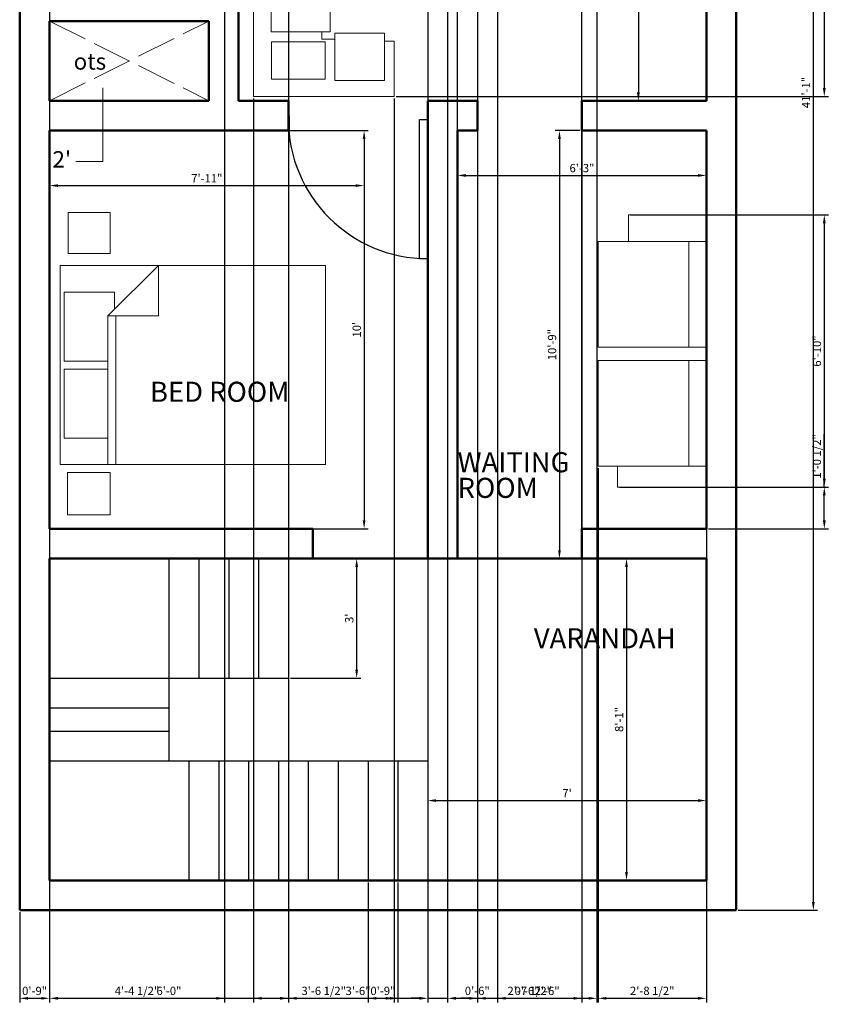
# Model space of a CAD drawing. Units: inches. Extents: x 1071 to 1348, y 2363 to 2916.
# Tile 1 of 4: x 1103 to 1348, y 2363 to 2660. Entities that reach past the tile are written whole.
import ezdxf

# ---------------------------------------------------------------- set-up
doc = ezdxf.new("R2010")
doc.units = ezdxf.units.IN
doc.linetypes.add('ACAD_ISO02W100', pattern=[15, 12, -3])
for name, color, linetype, lineweight in [('A-ANNO-DIMS', 2, 'Continuous', 18), ('A-ANNO-TEXT', 7, 'Continuous', 18), ('A-AREA-IDEN', 7, 'Continuous', 25), ('A-DOOR', 4, 'Continuous', 25), ('A-FLOR-OPEN', 8, 'ACAD_ISO02W100', 13), ('A-FLOR-STRS', 7, 'Continuous', 25), ('A-FURN', 8, 'Continuous', 18), ('A-WALL', 7, 'Continuous', 50)]:
    doc.layers.add(name, color=color, linetype=linetype, lineweight=lineweight)
doc.styles.get("Standard").update_dxf_attribs({"font": 'arial.ttf'})
doc.dimstyles.new('ISO-25', dxfattribs={"dimtxt": 2.5, "dimasz": 2.5, "dimexe": 1.25, "dimexo": 0.625, "dimtad": 1, "dimdec": 0, "dimlunit": 3, "dimtxsty": 'Standard', "dimcen": 2.5, "dimadec": 0, "dimazin": 0, "dimtfac": 1, "dimtdec": 0, "dimtmove": 0, "dimatfit": 3, "dimfxl": 1, "dimarcsym": 0})

# ---------------------------------------------------------------- blocks, each defined once
blk = doc.blocks.new('*U2')
for p, q in [((0, 0), (0, -100)), ((750, 0), (750, -100))]:
    blk.add_line(p, q)
blk.add_lwpolyline([(0, 0), (0, 750), (43.75, 750), (43.75, 0)], close=True)
blk.add_arc((0, 0), 750, 0, 90)
blk = doc.blocks.new('Bed - Queen')
for p, q in [((0, -80.00003), (0, 0)), ((0, 0), (59.99999, 0)), ((59.99999, 0), (59.99999, -80.00003)), ((7.99999, -1.2), (28.79998, -1.2)), ((7.99999, -14.4), (7.99999, -1.2)), ((28.79998, -1.2), (28.79998, -14.4)), ((31.19999, -1.2), (51.99999, -1.2)), ((31.19999, -14.4), (31.19999, -1.2)), ((51.99999, -1.2), (51.99999, -16.4)), ((0, -14.4), (44.8, -14.4)), ((59.99999, -29.6), (44.8, -14.4)), ((44.8, -14.4), (44.8, -29.6)), ((44.8, -16.8), (0, -16.8)), ((51.99999, -16.4), (46.79936, -16.4)), ((44.8, -29.6), (59.99999, -29.6)), ((59.99999, -80.00003), (0, -80.00003))]:
    blk.add_line(p, q)
blk = doc.blocks.new('*D10')
at = {"layer": 'A-ANNO-DIMS', "color": 0, "lineweight": -2, "transparency": 16777216}
for p, q in [((1184.91, 2497.25), (1206.11, 2497.25)), ((1204.86, 2494.75), (1204.86, 2463.75)), ((1184.91, 2461.25), (1206.11, 2461.25))]:
    blk.add_line(p, q, dxfattribs=at)
at = {"layer": 'A-ANNO-DIMS', "color": 0, "transparency": 16777216}
for points in [[(1204.45, 2494.75), (1205.28, 2494.75), (1204.86, 2497.25)], [(1204.45, 2463.75), (1205.28, 2463.75), (1204.86, 2461.25)]]:
    blk.add_solid(points, dxfattribs=at)
at = {"layer": 'Defpoints', "color": 0, "transparency": 16777216}
for p in [(1184.28, 2497.25), (1184.28, 2461.25), (1204.86, 2461.25)]:
    blk.add_point(p, dxfattribs=at)
at = {"layer": 'A-ANNO-DIMS', "color": 0, "transparency": 16777216, "insert": (1202.96, 2479.25), "char_height": 2.5, "attachment_point": 5, "rotation": 90}
blk.add_mtext("3'", dxfattribs=at)
blk = doc.blocks.new('*D11')
at = {"layer": 'A-ANNO-DIMS', "color": 0, "lineweight": -2, "transparency": 16777216}
for p, q in [((1235.28, 2607.11), (1235.28, 2613.98)), ((1237.78, 2612.73), (1307.78, 2612.73)), ((1310.28, 2607.11), (1310.28, 2613.98))]:
    blk.add_line(p, q, dxfattribs=at)
at = {"layer": 'A-ANNO-DIMS', "color": 0, "transparency": 16777216}
for points in [[(1237.78, 2613.15), (1237.78, 2612.32), (1235.28, 2612.73)], [(1307.78, 2613.15), (1307.78, 2612.32), (1310.28, 2612.73)]]:
    blk.add_solid(points, dxfattribs=at)
at = {"layer": 'Defpoints', "color": 0, "transparency": 16777216}
for p in [(1310.28, 2612.73), (1235.28, 2606.48), (1310.28, 2606.48)]:
    blk.add_point(p, dxfattribs=at)
at = {"layer": 'A-ANNO-DIMS', "color": 0, "transparency": 16777216, "insert": (1272.78, 2614.63), "char_height": 2.5, "attachment_point": 5}
blk.add_mtext('6\'-3"', dxfattribs=at)
blk = doc.blocks.new('*D12')
at = {"layer": 'A-ANNO-DIMS', "color": 0, "lineweight": -2, "transparency": 16777216}
for p, q in [((1272.16, 2626.25), (1264.74, 2626.25)), ((1265.99, 2623.75), (1265.99, 2499.75)), ((1272.16, 2497.25), (1264.74, 2497.25))]:
    blk.add_line(p, q, dxfattribs=at)
at = {"layer": 'A-ANNO-DIMS', "color": 0, "transparency": 16777216}
for points in [[(1265.58, 2623.75), (1266.41, 2623.75), (1265.99, 2626.25)], [(1265.58, 2499.75), (1266.41, 2499.75), (1265.99, 2497.25)]]:
    blk.add_solid(points, dxfattribs=at)
at = {"layer": 'Defpoints', "color": 0, "transparency": 16777216}
for p in [(1272.78, 2626.25), (1265.99, 2497.25), (1272.78, 2497.25)]:
    blk.add_point(p, dxfattribs=at)
at = {"layer": 'A-ANNO-DIMS', "color": 0, "transparency": 16777216, "insert": (1264.09, 2561.75), "char_height": 2.5, "attachment_point": 5, "rotation": 90}
blk.add_mtext('10\'-9"', dxfattribs=at)
blk = doc.blocks.new('*D13')
at = {"layer": 'A-ANNO-DIMS', "color": 0, "lineweight": -2, "transparency": 16777216}
for p, q in [((1293.16, 2746.25), (1288.53, 2746.25)), ((1289.78, 2743.75), (1289.78, 2637.75)), ((1290.91, 2635.25), (1288.53, 2635.25))]:
    blk.add_line(p, q, dxfattribs=at)
at = {"layer": 'A-ANNO-DIMS', "color": 0, "transparency": 16777216}
for points in [[(1289.36, 2743.75), (1290.19, 2743.75), (1289.78, 2746.25)], [(1289.36, 2637.75), (1290.19, 2637.75), (1289.78, 2635.25)]]:
    blk.add_solid(points, dxfattribs=at)
at = {"layer": 'Defpoints', "color": 0, "transparency": 16777216}
for p in [(1293.78, 2746.25), (1289.78, 2635.25), (1291.53, 2635.25)]:
    blk.add_point(p, dxfattribs=at)
at = {"layer": 'A-ANNO-DIMS', "color": 0, "transparency": 16777216, "insert": (1287.87, 2690.75), "char_height": 2.5, "attachment_point": 5, "rotation": 90}
blk.add_mtext('9\'-3"', dxfattribs=at)
blk = doc.blocks.new('*D15')
at = {"layer": 'A-ANNO-DIMS', "color": 0, "lineweight": -2, "transparency": 16777216}
for p, q in [((1171.71, 2626.25), (1208.36, 2626.25)), ((1207.11, 2623.75), (1207.11, 2508.75)), ((1171.71, 2506.25), (1208.36, 2506.25))]:
    blk.add_line(p, q, dxfattribs=at)
at = {"layer": 'A-ANNO-DIMS', "color": 0, "transparency": 16777216}
for points in [[(1206.69, 2623.75), (1207.52, 2623.75), (1207.11, 2626.25)], [(1206.69, 2508.75), (1207.52, 2508.75), (1207.11, 2506.25)]]:
    blk.add_solid(points, dxfattribs=at)
at = {"layer": 'Defpoints', "color": 0, "transparency": 16777216}
for p in [(1171.09, 2626.25), (1171.09, 2506.25), (1207.11, 2506.25)]:
    blk.add_point(p, dxfattribs=at)
at = {"layer": 'A-ANNO-DIMS', "color": 0, "transparency": 16777216, "insert": (1205.2, 2566.25), "char_height": 2.5, "attachment_point": 5, "rotation": 90}
blk.add_mtext("10'", dxfattribs=at)
blk = doc.blocks.new('*D16')
at = {"layer": 'A-ANNO-DIMS', "color": 0, "lineweight": -2, "transparency": 16777216}
for p, q in [((1290.65, 2497.25), (1284.96, 2497.25)), ((1286.21, 2494.75), (1286.21, 2402.75)), ((1290.65, 2400.25), (1284.96, 2400.25))]:
    blk.add_line(p, q, dxfattribs=at)
at = {"layer": 'A-ANNO-DIMS', "color": 0, "transparency": 16777216}
for points in [[(1285.79, 2494.75), (1286.62, 2494.75), (1286.21, 2497.25)], [(1285.79, 2402.75), (1286.62, 2402.75), (1286.21, 2400.25)]]:
    blk.add_solid(points, dxfattribs=at)
at = {"layer": 'Defpoints', "color": 0, "transparency": 16777216}
for p in [(1291.27, 2497.25), (1286.21, 2400.25), (1291.27, 2400.25)]:
    blk.add_point(p, dxfattribs=at)
at = {"layer": 'A-ANNO-DIMS', "color": 0, "transparency": 16777216, "insert": (1284.31, 2448.75), "char_height": 2.5, "attachment_point": 5, "rotation": 90}
blk.add_mtext('8\'-1"', dxfattribs=at)
blk = doc.blocks.new('*D17')
at = {"layer": 'A-ANNO-DIMS', "color": 0, "lineweight": -2, "transparency": 16777216}
for p, q in [((1226.28, 2435.63), (1226.28, 2423.06)), ((1310.28, 2435.63), (1310.28, 2423.06)), ((1228.78, 2424.31), (1307.78, 2424.31))]:
    blk.add_line(p, q, dxfattribs=at)
at = {"layer": 'A-ANNO-DIMS', "color": 0, "transparency": 16777216}
for points in [[(1228.78, 2424.72), (1228.78, 2423.89), (1226.28, 2424.31)], [(1307.78, 2424.72), (1307.78, 2423.89), (1310.28, 2424.31)]]:
    blk.add_solid(points, dxfattribs=at)
at = {"layer": 'Defpoints', "color": 0, "transparency": 16777216}
for p in [(1226.28, 2436.25), (1310.28, 2436.25), (1310.28, 2424.31)]:
    blk.add_point(p, dxfattribs=at)
at = {"layer": 'A-ANNO-DIMS', "color": 0, "transparency": 16777216, "insert": (1268.28, 2426.18), "char_height": 2.5, "attachment_point": 5}
blk.add_mtext("7'", dxfattribs=at)
blk = doc.blocks.new('*D18')
at = {"layer": 'A-ANNO-DIMS', "color": 0, "lineweight": -2, "transparency": 16777216}
for p, q in [((1112.28, 2609.69), (1112.28, 2608.43)), ((1114.78, 2609.68), (1204.61, 2609.68)), ((1207.11, 2609.69), (1207.11, 2608.43))]:
    blk.add_line(p, q, dxfattribs=at)
at = {"layer": 'A-ANNO-DIMS', "color": 0, "transparency": 16777216}
for points in [[(1114.78, 2610.09), (1114.78, 2609.26), (1112.28, 2609.68)], [(1204.61, 2610.09), (1204.61, 2609.26), (1207.11, 2609.68)]]:
    blk.add_solid(points, dxfattribs=at)
at = {"layer": 'Defpoints', "color": 0, "transparency": 16777216}
for p in [(1112.28, 2610.31), (1207.11, 2610.31), (1207.11, 2609.68)]:
    blk.add_point(p, dxfattribs=at)
at = {"layer": 'A-ANNO-DIMS', "color": 0, "transparency": 16777216, "insert": (1159.69, 2611.56), "char_height": 2.5, "attachment_point": 5}
blk.add_mtext('7\'-11"', dxfattribs=at)
blk = doc.blocks.new('*D21')
at = {"layer": 'A-ANNO-DIMS', "color": 0, "lineweight": -2, "transparency": 16777216}
for p, q in [((1319.91, 2884.25), (1343.77, 2884.25)), ((1342.52, 2881.75), (1342.52, 2393.75)), ((1319.91, 2391.25), (1343.77, 2391.25))]:
    blk.add_line(p, q, dxfattribs=at)
at = {"layer": 'A-ANNO-DIMS', "color": 0, "transparency": 16777216}
for points in [[(1342.11, 2881.75), (1342.94, 2881.75), (1342.52, 2884.25)], [(1342.11, 2393.75), (1342.94, 2393.75), (1342.52, 2391.25)]]:
    blk.add_solid(points, dxfattribs=at)
at = {"layer": 'Defpoints', "color": 0, "transparency": 16777216}
for p in [(1319.28, 2884.25), (1319.28, 2391.25), (1342.52, 2391.25)]:
    blk.add_point(p, dxfattribs=at)
at = {"layer": 'A-ANNO-DIMS', "color": 0, "transparency": 16777216, "insert": (1340.64, 2637.75), "char_height": 2.5, "attachment_point": 5, "rotation": 90}
blk.add_mtext('41\'-1"', dxfattribs=at)
blk = doc.blocks.new('NIGHTSTAND-A')
blk.add_lwpolyline([(0, 12.88), (12.76, 12.88), (12.76, 0), (0, 0)], close=True)
blk = doc.blocks.new('NIGHTSTAND-B')
blk.add_lwpolyline([(0, 0), (12.33, 0), (12.33, 12.6), (0, 12.6)], close=True)
blk = doc.blocks.new('*D45')
at = {"layer": 'A-ANNO-DIMS', "color": 0, "lineweight": -2, "transparency": 16777216}
for p, q in [((1112.28, 2634.63), (1112.28, 2363.45)), ((1184.28, 2634.63), (1184.28, 2363.45)), ((1114.78, 2364.7), (1181.78, 2364.7))]:
    blk.add_line(p, q, dxfattribs=at)
at = {"layer": 'A-ANNO-DIMS', "color": 0, "transparency": 16777216}
for points in [[(1114.78, 2365.12), (1114.78, 2364.29), (1112.28, 2364.7)], [(1181.78, 2365.12), (1181.78, 2364.29), (1184.28, 2364.7)]]:
    blk.add_solid(points, dxfattribs=at)
at = {"layer": 'Defpoints', "color": 0, "transparency": 16777216}
for p in [(1112.28, 2635.25), (1184.28, 2635.25), (1184.28, 2364.7)]:
    blk.add_point(p, dxfattribs=at)
at = {"layer": 'A-ANNO-DIMS', "color": 0, "transparency": 16777216, "insert": (1148.28, 2366.61), "char_height": 2.5, "attachment_point": 5}
blk.add_mtext('6\'-0"', dxfattribs=at)
blk = doc.blocks.new('*D46')
at = {"layer": 'A-ANNO-DIMS', "color": 0, "lineweight": -2, "transparency": 16777216}
for p, q in [((1184.28, 2634.63), (1184.28, 2363.45)), ((1226.28, 2634.63), (1226.28, 2363.45)), ((1186.78, 2364.7), (1223.78, 2364.7))]:
    blk.add_line(p, q, dxfattribs=at)
at = {"layer": 'A-ANNO-DIMS', "color": 0, "transparency": 16777216}
for points in [[(1186.78, 2365.12), (1186.78, 2364.29), (1184.28, 2364.7)], [(1223.78, 2365.12), (1223.78, 2364.29), (1226.28, 2364.7)]]:
    blk.add_solid(points, dxfattribs=at)
at = {"layer": 'Defpoints', "color": 0, "transparency": 16777216}
for p in [(1184.28, 2635.25), (1226.28, 2635.25), (1226.28, 2364.7)]:
    blk.add_point(p, dxfattribs=at)
at = {"layer": 'A-ANNO-DIMS', "color": 0, "transparency": 16777216, "insert": (1205.28, 2366.61), "char_height": 2.5, "attachment_point": 5}
blk.add_mtext('3\'-6"', dxfattribs=at)
blk = doc.blocks.new('*D47')
at = {"layer": 'A-ANNO-DIMS', "color": 0, "lineweight": -2, "transparency": 16777216}
for p, q in [((1112.28, 2399.63), (1112.28, 2363.45)), ((1103.28, 2390.63), (1103.28, 2363.45)), ((1105.78, 2364.7), (1109.78, 2364.7))]:
    blk.add_line(p, q, dxfattribs=at)
at = {"layer": 'A-ANNO-DIMS', "color": 0, "transparency": 16777216}
for points in [[(1105.78, 2365.12), (1105.78, 2364.29), (1103.28, 2364.7)], [(1109.78, 2365.12), (1109.78, 2364.29), (1112.28, 2364.7)]]:
    blk.add_solid(points, dxfattribs=at)
at = {"layer": 'Defpoints', "color": 0, "transparency": 16777216}
for p in [(1112.28, 2400.25), (1103.28, 2391.25), (1112.28, 2364.7)]:
    blk.add_point(p, dxfattribs=at)
at = {"layer": 'A-ANNO-DIMS', "color": 0, "transparency": 16777216, "insert": (1107.78, 2366.61), "char_height": 2.5, "attachment_point": 5}
blk.add_mtext('0\'-9"', dxfattribs=at)
blk = doc.blocks.new('*D48')
at = {"layer": 'A-ANNO-DIMS', "color": 0, "lineweight": -2, "transparency": 16777216}
for p, q in [((1184.28, 2745.63), (1184.28, 2363.45)), ((1226.28, 2745.63), (1226.28, 2363.45)), ((1186.78, 2364.7), (1223.78, 2364.7))]:
    blk.add_line(p, q, dxfattribs=at)
at = {"layer": 'A-ANNO-DIMS', "color": 0, "transparency": 16777216}
for points in [[(1186.78, 2365.12), (1186.78, 2364.29), (1184.28, 2364.7)], [(1223.78, 2365.12), (1223.78, 2364.29), (1226.28, 2364.7)]]:
    blk.add_solid(points, dxfattribs=at)
at = {"layer": 'Defpoints', "color": 0, "transparency": 16777216}
for p in [(1184.28, 2746.25), (1226.28, 2746.25), (1226.28, 2364.7)]:
    blk.add_point(p, dxfattribs=at)
at = {"layer": 'A-ANNO-DIMS', "color": 0, "transparency": 16777216, "insert": (1205.28, 2366.61), "char_height": 2.5, "attachment_point": 5}
blk.add_mtext('3\'-6"', dxfattribs=at)
blk = doc.blocks.new('*D49')
at = {"layer": 'A-ANNO-DIMS', "color": 0, "lineweight": -2, "transparency": 16777216}
for p, q in [((1247.28, 2745.63), (1247.28, 2363.45)), ((1277.28, 2745.63), (1277.28, 2363.45)), ((1249.78, 2364.7), (1274.78, 2364.7))]:
    blk.add_line(p, q, dxfattribs=at)
at = {"layer": 'A-ANNO-DIMS', "color": 0, "transparency": 16777216}
for points in [[(1249.78, 2365.12), (1249.78, 2364.29), (1247.28, 2364.7)], [(1274.78, 2365.12), (1274.78, 2364.29), (1277.28, 2364.7)]]:
    blk.add_solid(points, dxfattribs=at)
at = {"layer": 'Defpoints', "color": 0, "transparency": 16777216}
for p in [(1247.28, 2746.25), (1277.28, 2746.25), (1277.28, 2364.7)]:
    blk.add_point(p, dxfattribs=at)
at = {"layer": 'A-ANNO-DIMS', "color": 0, "transparency": 16777216, "insert": (1262.28, 2366.61), "char_height": 2.5, "attachment_point": 5}
blk.add_mtext('2\'-6"', dxfattribs=at)
blk = doc.blocks.new('*D51')
at = {"layer": 'A-ANNO-DIMS', "color": 0, "lineweight": -2, "transparency": 16777216}
for p, q in [((1241.28, 2634.63), (1241.28, 2363.45)), ((1272.78, 2634.63), (1272.78, 2363.45)), ((1243.78, 2364.7), (1270.28, 2364.7))]:
    blk.add_line(p, q, dxfattribs=at)
at = {"layer": 'A-ANNO-DIMS', "color": 0, "transparency": 16777216}
for points in [[(1243.78, 2365.12), (1243.78, 2364.29), (1241.28, 2364.7)], [(1270.28, 2365.12), (1270.28, 2364.29), (1272.78, 2364.7)]]:
    blk.add_solid(points, dxfattribs=at)
at = {"layer": 'Defpoints', "color": 0, "transparency": 16777216}
for p in [(1241.28, 2635.25), (1272.78, 2635.25), (1272.78, 2364.7)]:
    blk.add_point(p, dxfattribs=at)
at = {"layer": 'A-ANNO-DIMS', "color": 0, "transparency": 16777216, "insert": (1257.03, 2366.62), "char_height": 2.5, "attachment_point": 5}
blk.add_mtext('2\'-7 1/2"', dxfattribs=at)
blk = doc.blocks.new('*D53')
at = {"layer": 'A-ANNO-DIMS', "color": 0, "lineweight": -2, "transparency": 16777216}
for p, q in [((1226.28, 2754.63), (1226.28, 2363.45)), ((1232.28, 2754.63), (1232.28, 2363.45)), ((1223.78, 2364.7), (1221.28, 2364.7)), ((1226.28, 2364.7), (1232.28, 2364.7)), ((1234.78, 2364.7), (1245.18, 2364.7))]:
    blk.add_line(p, q, dxfattribs=at)
at = {"layer": 'A-ANNO-DIMS', "color": 0, "transparency": 16777216}
for points in [[(1223.78, 2365.12), (1223.78, 2364.29), (1226.28, 2364.7)], [(1234.78, 2365.12), (1234.78, 2364.29), (1232.28, 2364.7)]]:
    blk.add_solid(points, dxfattribs=at)
at = {"layer": 'Defpoints', "color": 0, "transparency": 16777216}
for p in [(1226.28, 2755.25), (1232.28, 2755.25), (1232.28, 2364.7)]:
    blk.add_point(p, dxfattribs=at)
at = {"layer": 'A-ANNO-DIMS', "color": 0, "transparency": 16777216, "insert": (1241.23, 2366.61), "char_height": 2.5, "attachment_point": 5}
blk.add_mtext('0\'-6"', dxfattribs=at)
blk = doc.blocks.new('*D54')
at = {"layer": 'A-ANNO-DIMS', "color": 0, "lineweight": -2, "transparency": 16777216}
for p, q in [((1241.28, 2754.63), (1241.28, 2363.45)), ((1247.28, 2754.63), (1247.28, 2363.45)), ((1238.78, 2364.7), (1236.28, 2364.7)), ((1241.28, 2364.7), (1247.28, 2364.7)), ((1249.78, 2364.7), (1260.18, 2364.7))]:
    blk.add_line(p, q, dxfattribs=at)
at = {"layer": 'A-ANNO-DIMS', "color": 0, "transparency": 16777216}
for points in [[(1238.78, 2365.12), (1238.78, 2364.29), (1241.28, 2364.7)], [(1249.78, 2365.12), (1249.78, 2364.29), (1247.28, 2364.7)]]:
    blk.add_solid(points, dxfattribs=at)
at = {"layer": 'Defpoints', "color": 0, "transparency": 16777216}
for p in [(1241.28, 2755.25), (1247.28, 2755.25), (1247.28, 2364.7)]:
    blk.add_point(p, dxfattribs=at)
at = {"layer": 'A-ANNO-DIMS', "color": 0, "transparency": 16777216, "insert": (1256.23, 2366.61), "char_height": 2.5, "attachment_point": 5}
blk.add_mtext('0\'-6"', dxfattribs=at)
blk = doc.blocks.new('*D55')
at = {"layer": 'A-ANNO-DIMS', "color": 0, "lineweight": -2, "transparency": 16777216}
for p, q in [((1208.28, 2399.63), (1208.28, 2363.45)), ((1217.28, 2399.63), (1217.28, 2363.45)), ((1210.78, 2364.7), (1214.78, 2364.7))]:
    blk.add_line(p, q, dxfattribs=at)
at = {"layer": 'A-ANNO-DIMS', "color": 0, "transparency": 16777216}
for points in [[(1210.78, 2365.12), (1210.78, 2364.29), (1208.28, 2364.7)], [(1214.78, 2365.12), (1214.78, 2364.29), (1217.28, 2364.7)]]:
    blk.add_solid(points, dxfattribs=at)
at = {"layer": 'Defpoints', "color": 0, "transparency": 16777216}
for p in [(1208.28, 2400.25), (1217.28, 2400.25), (1217.28, 2364.7)]:
    blk.add_point(p, dxfattribs=at)
at = {"layer": 'A-ANNO-DIMS', "color": 0, "transparency": 16777216, "insert": (1212.78, 2366.61), "char_height": 2.5, "attachment_point": 5}
blk.add_mtext('0\'-9"', dxfattribs=at)
blk = doc.blocks.new('*D56')
at = {"layer": 'A-ANNO-DIMS', "color": 0, "lineweight": -2, "transparency": 16777216}
for p, q in [((1235.28, 2497.88), (1235.28, 2912.05)), ((1272.78, 2497.88), (1272.78, 2912.05)), ((1237.78, 2910.8), (1270.28, 2910.8))]:
    blk.add_line(p, q, dxfattribs=at)
at = {"layer": 'A-ANNO-DIMS', "color": 0, "transparency": 16777216}
for points in [[(1237.78, 2911.22), (1237.78, 2910.39), (1235.28, 2910.8)], [(1270.28, 2911.22), (1270.28, 2910.39), (1272.78, 2910.8)]]:
    blk.add_solid(points, dxfattribs=at)
at = {"layer": 'Defpoints', "color": 0, "transparency": 16777216}
for p in [(1272.78, 2910.8), (1235.28, 2497.25), (1272.78, 2497.25)]:
    blk.add_point(p, dxfattribs=at)
at = {"layer": 'A-ANNO-DIMS', "color": 0, "transparency": 16777216, "insert": (1254.03, 2912.72), "char_height": 2.5, "attachment_point": 5}
blk.add_mtext('3\'-1 1/2"', dxfattribs=at)
blk = doc.blocks.new('*D57')
at = {"layer": 'A-ANNO-DIMS', "color": 0, "lineweight": -2, "transparency": 16777216}
for p, q in [((1287.4, 2600.82), (1347.08, 2600.82)), ((1345.83, 2598.32), (1345.83, 2521.3)), ((1284.17, 2518.8), (1347.08, 2518.8))]:
    blk.add_line(p, q, dxfattribs=at)
at = {"layer": 'A-ANNO-DIMS', "color": 0, "transparency": 16777216}
for points in [[(1345.41, 2598.32), (1346.25, 2598.32), (1345.83, 2600.82)], [(1345.41, 2521.3), (1346.25, 2521.3), (1345.83, 2518.8)]]:
    blk.add_solid(points, dxfattribs=at)
at = {"layer": 'Defpoints', "color": 0, "transparency": 16777216}
for p in [(1286.78, 2600.82), (1283.54, 2518.8), (1345.83, 2518.8)]:
    blk.add_point(p, dxfattribs=at)
at = {"layer": 'A-ANNO-DIMS', "color": 0, "transparency": 16777216, "insert": (1343.93, 2559.81), "char_height": 2.5, "attachment_point": 5, "rotation": 90}
blk.add_mtext('6\'-10"', dxfattribs=at)
blk = doc.blocks.new('*D58')
at = {"layer": 'A-ANNO-DIMS', "color": 0, "lineweight": -2, "transparency": 16777216}
for p, q in [((1277.63, 2524.49), (1277.63, 2363.45)), ((1310.28, 2518.18), (1310.28, 2363.45)), ((1280.13, 2364.7), (1307.78, 2364.7))]:
    blk.add_line(p, q, dxfattribs=at)
at = {"layer": 'A-ANNO-DIMS', "color": 0, "transparency": 16777216}
for points in [[(1280.13, 2365.12), (1280.13, 2364.29), (1277.63, 2364.7)], [(1307.78, 2365.12), (1307.78, 2364.29), (1310.28, 2364.7)]]:
    blk.add_solid(points, dxfattribs=at)
at = {"layer": 'Defpoints', "color": 0, "transparency": 16777216}
for p in [(1277.63, 2525.12), (1310.28, 2518.8), (1310.28, 2364.7)]:
    blk.add_point(p, dxfattribs=at)
at = {"layer": 'A-ANNO-DIMS', "color": 0, "transparency": 16777216, "insert": (1293.96, 2366.62), "char_height": 2.5, "attachment_point": 5}
blk.add_mtext('2\'-8 1/2"', dxfattribs=at)
blk = doc.blocks.new('*D59')
at = {"layer": 'A-ANNO-DIMS', "color": 0, "lineweight": -2, "transparency": 16777216}
for p, q in [((1345.83, 2518.8), (1345.83, 2534.79)), ((1310.91, 2518.8), (1347.08, 2518.8)), ((1345.83, 2508.75), (1345.83, 2516.3)), ((1310.91, 2506.25), (1347.08, 2506.25))]:
    blk.add_line(p, q, dxfattribs=at)
at = {"layer": 'A-ANNO-DIMS', "color": 0, "transparency": 16777216}
for points in [[(1345.41, 2516.3), (1346.25, 2516.3), (1345.83, 2518.8)], [(1345.41, 2508.75), (1346.25, 2508.75), (1345.83, 2506.25)]]:
    blk.add_solid(points, dxfattribs=at)
at = {"layer": 'Defpoints', "color": 0, "transparency": 16777216}
for p in [(1310.28, 2518.8), (1345.83, 2518.8), (1310.28, 2506.25)]:
    blk.add_point(p, dxfattribs=at)
at = {"layer": 'A-ANNO-DIMS', "color": 0, "transparency": 16777216, "insert": (1343.91, 2528.04), "char_height": 2.5, "attachment_point": 5, "rotation": 90}
blk.add_mtext('1\'-0 1/2"', dxfattribs=at)
blk = doc.blocks.new('*D63')
at = {"layer": 'A-ANNO-DIMS', "color": 0, "lineweight": -2, "transparency": 16777216}
for p, q in [((1112.28, 2754.63), (1112.28, 2363.45)), ((1165.02, 2754.63), (1165.02, 2363.45)), ((1114.78, 2364.7), (1162.52, 2364.7))]:
    blk.add_line(p, q, dxfattribs=at)
at = {"layer": 'A-ANNO-DIMS', "color": 0, "transparency": 16777216}
for points in [[(1114.78, 2365.12), (1114.78, 2364.29), (1112.28, 2364.7)], [(1162.52, 2365.12), (1162.52, 2364.29), (1165.02, 2364.7)]]:
    blk.add_solid(points, dxfattribs=at)
at = {"layer": 'Defpoints', "color": 0, "transparency": 16777216}
for p in [(1112.28, 2755.25), (1165.02, 2755.25), (1165.02, 2364.7)]:
    blk.add_point(p, dxfattribs=at)
at = {"layer": 'A-ANNO-DIMS', "color": 0, "transparency": 16777216, "insert": (1138.65, 2366.62), "char_height": 2.5, "attachment_point": 5}
blk.add_mtext('4\'-4 1/2"', dxfattribs=at)
blk = doc.blocks.new('*D65')
at = {"layer": 'A-ANNO-DIMS', "color": 0, "lineweight": -2, "transparency": 16777216}
for p, q in [((1173.73, 2635.94), (1173.73, 2363.45)), ((1216.12, 2635.94), (1216.12, 2363.45)), ((1176.23, 2364.7), (1213.62, 2364.7))]:
    blk.add_line(p, q, dxfattribs=at)
at = {"layer": 'A-ANNO-DIMS', "color": 0, "transparency": 16777216}
for points in [[(1176.23, 2365.12), (1176.23, 2364.29), (1173.73, 2364.7)], [(1213.62, 2365.12), (1213.62, 2364.29), (1216.12, 2364.7)]]:
    blk.add_solid(points, dxfattribs=at)
at = {"layer": 'Defpoints', "color": 0, "transparency": 16777216}
for p in [(1173.73, 2636.57), (1216.12, 2636.57), (1216.12, 2364.7)]:
    blk.add_point(p, dxfattribs=at)
at = {"layer": 'A-ANNO-DIMS', "color": 0, "transparency": 16777216, "insert": (1194.93, 2366.62), "char_height": 2.5, "attachment_point": 5}
blk.add_mtext('3\'-6 1/2"', dxfattribs=at)
blk = doc.blocks.new('*D66')
at = {"layer": 'A-ANNO-DIMS', "color": 0, "lineweight": -2, "transparency": 16777216}
for p, q in [((1193.46, 2707.65), (1347.08, 2707.65)), ((1345.83, 2705.15), (1345.83, 2639.07)), ((1216.75, 2636.57), (1347.08, 2636.57))]:
    blk.add_line(p, q, dxfattribs=at)
at = {"layer": 'A-ANNO-DIMS', "color": 0, "transparency": 16777216}
for points in [[(1345.41, 2705.15), (1346.25, 2705.15), (1345.83, 2707.65)], [(1345.41, 2639.07), (1346.25, 2639.07), (1345.83, 2636.57)]]:
    blk.add_solid(points, dxfattribs=at)
at = {"layer": 'Defpoints', "color": 0, "transparency": 16777216}
for p in [(1192.84, 2707.65), (1216.12, 2636.57), (1345.83, 2636.57)]:
    blk.add_point(p, dxfattribs=at)
at = {"layer": 'A-ANNO-DIMS', "color": 0, "transparency": 16777216, "insert": (1343.93, 2672.11), "char_height": 2.5, "attachment_point": 5, "rotation": 90}
blk.add_mtext('5\'-11"', dxfattribs=at)

msp = doc.modelspace()

# ---------------------------------------------------------------- linework, layer by layer
at = {"layer": 'A-ANNO-TEXT'}
for p, q in [((1128.35, 2639.16), (1128.35, 2616.93)), ((1128.35, 2616.93), (1120.19, 2616.93))]:
    msp.add_line(p, q, dxfattribs=at)
at = {"layer": 'A-FLOR-OPEN'}
for p, q in [((1112.28, 2635.25), (1160.28, 2659.25)), ((1112.28, 2659.25), (1160.28, 2635.25))]:
    msp.add_line(p, q, dxfattribs=at)
at = {"layer": 'A-FLOR-STRS'}
for p, q in [((1148.28, 2497.25), (1148.28, 2436.25)), ((1157.28, 2497.25), (1157.28, 2461.25)), ((1166.28, 2497.25), (1166.28, 2461.25)), ((1175.28, 2497.25), (1175.28, 2461.25)), ((1184.28, 2497.25), (1184.28, 2461.25)), ((1112.28, 2461.25), (1184.28, 2461.25)), ((1112.28, 2452.25), (1148.28, 2452.25)), ((1112.28, 2445.25), (1148.28, 2445.25)), ((1112.28, 2436.25), (1226.28, 2436.25)), ((1154.28, 2436.25), (1154.28, 2400.25)), ((1163.28, 2436.25), (1163.28, 2400.25)), ((1172.28, 2436.25), (1172.28, 2400.25)), ((1181.28, 2436.25), (1181.28, 2400.25)), ((1190.28, 2436.25), (1190.28, 2400.25)), ((1199.28, 2436.25), (1199.28, 2400.25)), ((1208.28, 2436.25), (1208.28, 2400.25)), ((1217.28, 2436.25), (1217.28, 2400.25)), ((1226.28, 2436.25), (1226.28, 2400.25))]:
    msp.add_line(p, q, dxfattribs=at)
at = {"layer": 'A-FURN'}
for p, q in [((1194.39, 2655.98), (1194.39, 2653.84)), ((1194.39, 2653.84), (1198.3, 2653.84)), ((1304.98, 2592.79), (1304.98, 2560.96)), ((1277.63, 2560.96), (1310.28, 2560.96)), ((1277.63, 2556.96), (1310.28, 2556.96)), ((1304.98, 2556.96), (1304.98, 2525.12))]:
    msp.add_line(p, q, dxfattribs=at)
for points in [[(1173.73, 2638.54), (1173.73, 2707.65), (1192.84, 2707.65), (1192.84, 2703.25)], [(1213.29, 2653.24), (1216.12, 2653.24), (1216.12, 2636.57), (1173.73, 2636.57), (1173.73, 2653.24)], [(1277.63, 2560.96), (1277.63, 2592.79), (1310.28, 2592.79), (1310.28, 2525.12), (1277.63, 2525.12), (1277.63, 2556.96)]]:
    msp.add_lwpolyline(points, dxfattribs=at)
for points in [[(1179.12, 2655.98), (1196.89, 2655.98), (1196.89, 2668.91), (1179.12, 2668.91)], [(1213.29, 2641.35), (1198.3, 2641.35), (1198.3, 2655.63), (1213.29, 2655.63)], [(1195.41, 2641.77), (1179.22, 2641.77), (1179.22, 2652.98), (1195.41, 2652.98)], [(1286.78, 2592.79), (1310.28, 2592.79), (1310.28, 2600.82), (1286.78, 2600.82)], [(1283.54, 2525.12), (1310.28, 2525.12), (1310.28, 2518.8), (1283.54, 2518.8)]]:
    msp.add_lwpolyline(points, close=True, dxfattribs=at)
at = {"layer": 'A-WALL'}
for p, q in [((1103.28, 2884.25), (1103.28, 2391.25)), ((1319.28, 2884.25), (1319.28, 2391.25)), ((1310.28, 2746.25), (1310.28, 2635.25)), ((1169.28, 2710.25), (1169.28, 2635.25)), ((1112.28, 2659.25), (1160.28, 2659.25)), ((1112.28, 2659.25), (1112.28, 2635.25)), ((1160.28, 2659.25), (1160.28, 2635.25)), ((1112.28, 2635.25), (1160.28, 2635.25)), ((1169.28, 2635.25), (1184.28, 2635.25)), ((1184.42, 2626.25), (1184.28, 2635.25)), ((1226.28, 2635.25), (1226.28, 2497.25)), ((1226.28, 2635.25), (1241.28, 2635.25)), ((1241.28, 2626.25), (1241.28, 2635.25)), ((1272.78, 2626.25), (1272.78, 2635.25)), ((1272.78, 2635.25), (1310.28, 2635.25)), ((1184.28, 2632.45), (1184.28, 2626.25)), ((1112.28, 2626.25), (1184.42, 2626.25)), ((1112.28, 2626.25), (1112.28, 2506.25)), ((1235.28, 2626.25), (1235.28, 2497.25)), ((1235.28, 2626.25), (1241.28, 2626.25)), ((1272.78, 2626.25), (1310.28, 2626.25)), ((1310.28, 2626.25), (1310.28, 2506.25)), ((1112.28, 2506.25), (1184.28, 2506.25)), ((1184.28, 2506.25), (1191.62, 2506.25)), ((1191.62, 2506.25), (1191.62, 2497.25)), ((1272.78, 2506.25), (1310.28, 2506.25)), ((1272.78, 2506.25), (1272.78, 2497.25)), ((1112.28, 2497.25), (1235.28, 2497.25)), ((1112.28, 2497.25), (1112.28, 2400.25)), ((1235.28, 2497.25), (1310.28, 2497.25)), ((1310.28, 2497.25), (1310.28, 2400.25)), ((1112.28, 2400.25), (1310.28, 2400.25)), ((1235.28, 2400.25), (1310.28, 2400.25)), ((1103.28, 2391.25), (1319.28, 2391.25))]:
    msp.add_line(p, q, dxfattribs=at)

# ---------------------------------------------------------------- block references
at = {"layer": 'A-DOOR', "xscale": 0.0559999999999998, "yscale": 0.0559999999999998, "zscale": 0.0559999999999998, "rotation": 180}
msp.add_blockref('*U2', (1226.28, 2629.65), dxfattribs=at)
at = {"layer": 'A-FURN'}
for name, p, rotation in [('NIGHTSTAND-B', (1130.54, 2589.24), 90.00000000000175), ('Bed - Queen', (1115.49, 2525.58), 90), ('NIGHTSTAND-A', (1130.54, 2510.43), 90.00000000000003)]:
    msp.add_blockref(name, p, dxfattribs=dict(at, rotation=rotation))

# ---------------------------------------------------------------- texts
at = {"layer": 'A-ANNO-TEXT'}
msp.add_text("2'", height=4.936, dxfattribs=at).set_placement((1113.17, 2615.13))
at = {"layer": 'A-AREA-IDEN'}
for s, height, p in [('ots', 4.936, (1119.56, 2644.63)), ('BED ROOM', 6.055, (1142.56, 2544.5)), ('WAITING', 6.055, (1235.28, 2523.27)), ('ROOM', 6.055, (1235.28, 2515.54)), ('VARANDAH', 6.055, (1258.27, 2470.2))]:
    msp.add_text(s, height=height, dxfattribs=at).set_placement(p)

# ---------------------------------------------------------------- dimensions: what is measured, and where the dimension line sits
at = {"layer": 'A-ANNO-DIMS'}
for base, p1, p2, override, picture, middle in [((1272.78, 2910.8), (1235.28, 2497.25), (1272.78, 2497.25), {"dimdec": 1, "dimlfac": 1, "dimrnd": 0, "dimzin": 1, "dimdsep": 46, "dimlunit": 4, "dimfrac": 2}, '*D56', (1254.03, 2912.72)), ((1165.02, 2364.7), (1112.28, 2755.25), (1165.02, 2755.25), {"dimdec": 1, "dimlfac": 1, "dimrnd": 0, "dimzin": 1, "dimdsep": 46, "dimlunit": 4, "dimfrac": 2}, '*D63', (1138.65, 2366.62)), ((1232.28, 2364.7), (1226.28, 2755.25), (1232.28, 2755.25), {"dimdec": 1, "dimlfac": 1, "dimrnd": 0, "dimzin": 1, "dimdsep": 46, "dimlunit": 4, "dimfrac": 2}, '*D53', (1241.23, 2366.61)), ((1247.28, 2364.7), (1241.28, 2755.25), (1247.28, 2755.25), {"dimdec": 1, "dimlfac": 1, "dimrnd": 0, "dimzin": 1, "dimdsep": 46, "dimlunit": 4, "dimfrac": 2}, '*D54', (1256.23, 2366.61)), ((1226.28, 2364.7), (1184.28, 2746.25), (1226.28, 2746.25), {"dimdec": 1, "dimlfac": 1, "dimrnd": 0, "dimzin": 1, "dimdsep": 46, "dimlunit": 4, "dimfrac": 2}, '*D48', (1205.28, 2366.61)), ((1277.28, 2364.7), (1247.28, 2746.25), (1277.28, 2746.25), {"dimdec": 1, "dimlfac": 1, "dimrnd": 0, "dimzin": 1, "dimdsep": 46, "dimlunit": 4, "dimfrac": 2}, '*D49', (1262.28, 2366.61)), ((1216.12, 2364.7), (1173.73, 2636.57), (1216.12, 2636.57), {"dimdec": 1, "dimlfac": 1, "dimrnd": 0, "dimzin": 1, "dimdsep": 46, "dimlunit": 4, "dimfrac": 2}, '*D65', (1194.93, 2366.62)), ((1184.28, 2364.7), (1112.28, 2635.25), (1184.28, 2635.25), {"dimdec": 1, "dimlfac": 1, "dimrnd": 0, "dimzin": 1, "dimdsep": 46, "dimlunit": 4, "dimfrac": 2}, '*D45', (1148.28, 2366.61)), ((1226.28, 2364.7), (1184.28, 2635.25), (1226.28, 2635.25), {"dimdec": 1, "dimlfac": 1, "dimrnd": 0, "dimzin": 1, "dimdsep": 46, "dimlunit": 4, "dimfrac": 2}, '*D46', (1205.28, 2366.61)), ((1272.78, 2364.7), (1241.28, 2635.25), (1272.78, 2635.25), {"dimdec": 1, "dimlfac": 1, "dimrnd": 0, "dimzin": 1, "dimdsep": 46, "dimlunit": 4, "dimfrac": 2}, '*D51', (1257.03, 2366.62)), ((1310.28, 2612.73), (1235.28, 2606.48), (1310.28, 2606.48), {"dimclrd": 0, "dimclre": 0, "dimclrt": 0}, '*D11', (1272.78, 2614.63)), ((1207.11, 2609.68), (1112.28, 2610.31), (1207.11, 2610.31), {"dimclrd": 0, "dimclre": 0, "dimclrt": 0}, '*D18', (1159.69, 2611.56)), ((1310.281, 2364.7048), (1277.6329, 2525.119), (1310.281, 2518.8), {"dimdec": 1, "dimlfac": 1, "dimrnd": 0, "dimzin": 1, "dimdsep": 46, "dimlunit": 4, "dimfrac": 2}, '*D58', (1293.9569, 2366.6224)), ((1310.28, 2424.31), (1226.28, 2436.25), (1310.28, 2436.25), {"dimclrd": 0, "dimclre": 0, "dimclrt": 0}, '*D17', (1268.28, 2426.18)), ((1112.28, 2364.7), (1103.28, 2391.25), (1112.28, 2400.25), {"dimdec": 1, "dimlfac": 1, "dimrnd": 0, "dimzin": 1, "dimdsep": 46, "dimlunit": 4, "dimfrac": 2}, '*D47', (1107.78, 2366.61)), ((1217.28, 2364.7), (1208.28, 2400.25), (1217.28, 2400.25), {"dimdec": 1, "dimlfac": 1, "dimrnd": 0, "dimzin": 1, "dimdsep": 46, "dimlunit": 4, "dimfrac": 2}, '*D55', (1212.78, 2366.61))]:
    dim = msp.add_linear_dim(base=base, p1=p1, p2=p2, dimstyle='ISO-25', override=override, dxfattribs=at)
    dim.commit()
    dim.dimension.update_dxf_attribs({"geometry": picture, "text_midpoint": middle})
for base, p1, p2, override, picture, middle in [((1342.52, 2391.25), (1319.28, 2884.25), (1319.28, 2391.25), {"dimclrd": 0, "dimclre": 0, "dimclrt": 0}, '*D21', (1340.64, 2637.75)), ((1289.78, 2635.25), (1293.78, 2746.25), (1291.53, 2635.25), {"dimclrd": 0, "dimclre": 0, "dimclrt": 0}, '*D13', (1287.87, 2690.75)), ((1345.83, 2636.57), (1192.84, 2707.65), (1216.12, 2636.57), {"dimdec": 1, "dimlfac": 1, "dimrnd": 0, "dimzin": 1, "dimdsep": 46, "dimlunit": 4, "dimfrac": 2}, '*D66', (1343.93, 2672.11)), ((1207.11, 2506.25), (1171.09, 2626.25), (1171.09, 2506.25), {"dimclrd": 0, "dimclre": 0, "dimclrt": 0}, '*D15', (1205.2, 2566.25)), ((1265.99, 2497.25), (1272.78, 2626.25), (1272.78, 2497.25), {"dimclrd": 0, "dimclre": 0, "dimclrt": 0}, '*D12', (1264.09, 2561.75)), ((1345.83, 2518.8), (1286.78, 2600.82), (1283.54, 2518.8), {"dimdec": 1, "dimlfac": 1, "dimrnd": 0, "dimzin": 1, "dimdsep": 46, "dimlunit": 4, "dimfrac": 2}, '*D57', (1343.93, 2559.81)), ((1345.831, 2518.8), (1310.281, 2506.2548), (1310.281, 2518.8), {"dimdec": 1, "dimlfac": 1, "dimrnd": 0, "dimzin": 1, "dimdsep": 46, "dimlunit": 4, "dimfrac": 2}, '*D59', (1343.9133, 2528.0429)), ((1204.86, 2461.25), (1184.28, 2497.25), (1184.28, 2461.25), {"dimclrd": 0, "dimclre": 0, "dimclrt": 0}, '*D10', (1202.96, 2479.25)), ((1286.21, 2400.25), (1291.27, 2497.25), (1291.27, 2400.25), {"dimclrd": 0, "dimclre": 0, "dimclrt": 0}, '*D16', (1284.31, 2448.75))]:
    dim = msp.add_linear_dim(base=base, p1=p1, p2=p2, angle=90, dimstyle='ISO-25', override=override, dxfattribs=at)
    dim.commit()
    dim.dimension.update_dxf_attribs({"geometry": picture, "text_midpoint": middle})

doc.saveas('drawing.dxf')
